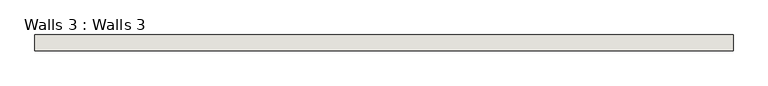
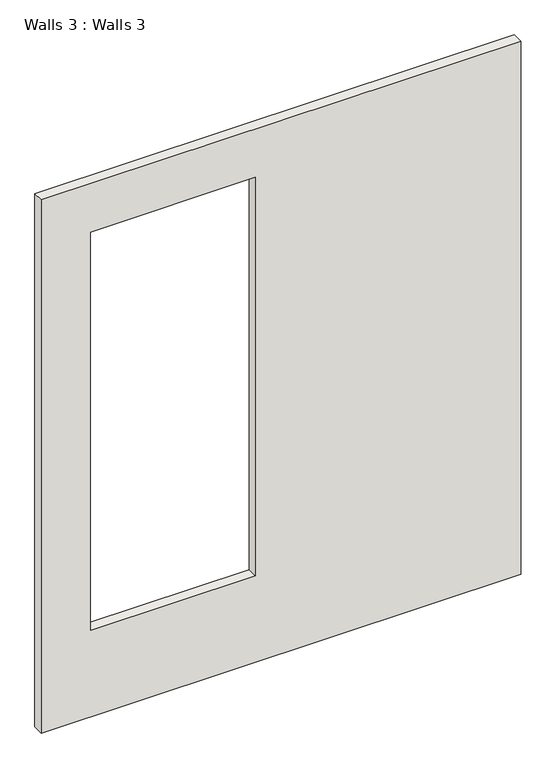
"""IFC4 building model written with IfcOpenShell, lengths in millimetres: wall geometry, Walls 3 : Walls 3."""

from ifc_helpers import new_model, si_unit, frame, origin, place, context, project, spatial, polyline, outline, extrude, source, transform, mapped, element, save


def walls_3_walls_3_f969b8b6(model_context):
    return source(origin(), model_context, "Body", "SweptSolid", [
        extrude(outline(polyline([(6587.697392, -1871.6311901), (6587.697392, -7474.5150201), (0.0, -7474.5150201), (0.0, -1871.6311901), (6587.697392, -1871.6311901)]), holes=[polyline([(5988.5853432, -4972.3150386), (1066.8, -4972.3150386), (1066.8, -6896.7101003), (5988.5853432, -6896.7101003), (5988.5853432, -4972.3150386)])]), frame((0.0, -4372.4106756, 0.0), z_axis=(0.0, 1.0, 0.0), x_axis=(0.0, 0.0, 1.0)), (0.0, 0.0, 1.0), 126.6967244),
    ])


if __name__ == "__main__":
    model = new_model("IFC4")
    model_context = context("Model", 3, world=origin())
    ifc_project = project(units=[si_unit("LENGTHUNIT", "METRE", prefix="MILLI")], contexts=[model_context])
    site = spatial("IfcSite", under=ifc_project)
    building = spatial("IfcBuilding", under=site)
    placement = place(None, origin())
    walls_3_walls_3_shape = walls_3_walls_3_f969b8b6(model_context)
    element("IfcWall", 1, ObjectType="Walls 3 : Walls 3", at=placement, inside=building, context=model_context, shape_type="MappedRepresentation", body=[
        mapped(walls_3_walls_3_shape, transform((0.0, 0.0, 0.0), x_axis=(1.0, 0.0, 0.0), y_axis=(0.0, 1.0, 0.0), z_axis=(0.0, 0.0, 1.0))),
    ])
    save(model, "model.ifc")

# Revit data of these elements
# Element 1 (IfcWall, "Walls 3 : Walls 3")
#   Materials on its faces: "Default Wall"
# Materials
#   "Default Wall": colour RGB 128 128 128, transparency 0
